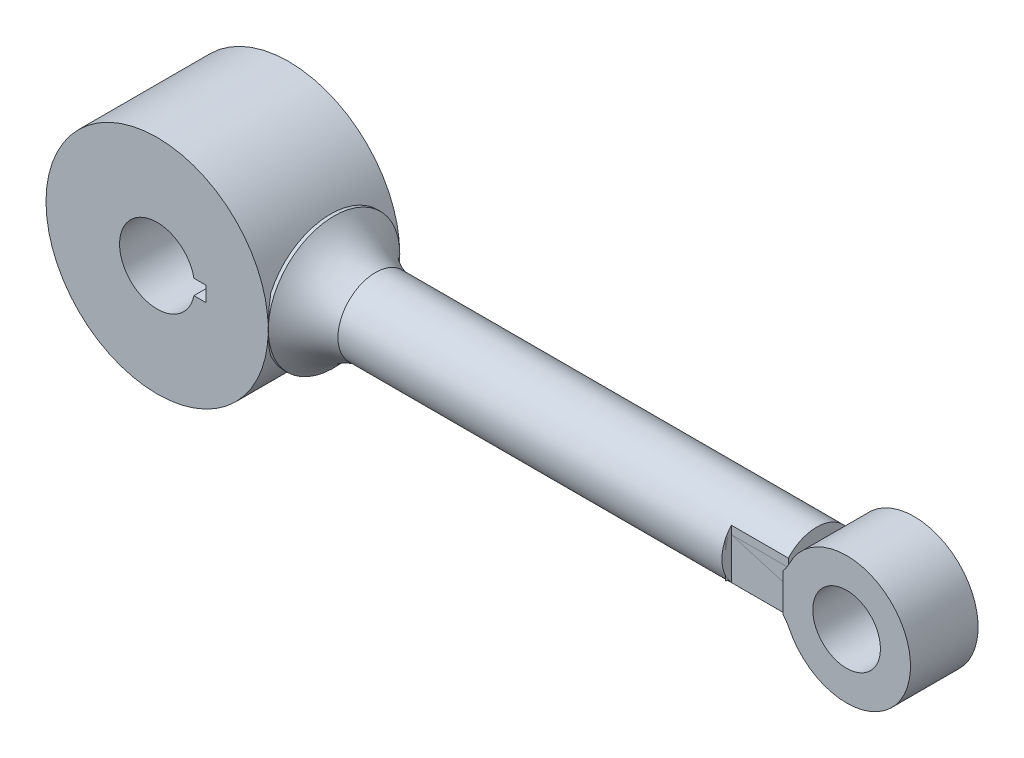
ISO-10303-21;
HEADER;
FILE_DESCRIPTION(('STEP AP214'),'2;1');
FILE_NAME('part.step','',(''),(''),'','','');
FILE_SCHEMA(('AUTOMOTIVE_DESIGN { 1 0 10303 214 1 1 1 1 }'));
ENDSEC;
DATA;
#1=APPLICATION_CONTEXT('core data for automotive mechanical design processes');
#2=APPLICATION_PROTOCOL_DEFINITION('international standard','automotive_design',2000,#1);
#3=PRODUCT_CONTEXT('',#1,'mechanical');
#4=PRODUCT('Part','Part','',(#3));
#5=PRODUCT_RELATED_PRODUCT_CATEGORY('part','',(#4));
#6=PRODUCT_DEFINITION_FORMATION('','',#4);
#7=PRODUCT_DEFINITION_CONTEXT('part definition',#1,'design');
#8=PRODUCT_DEFINITION('design','',#6,#7);
#9=PRODUCT_DEFINITION_SHAPE('','',#8);
#10=(LENGTH_UNIT() NAMED_UNIT(*) SI_UNIT(.MILLI.,.METRE.));
#11=(NAMED_UNIT(*) PLANE_ANGLE_UNIT() SI_UNIT($,.RADIAN.));
#12=(NAMED_UNIT(*) SI_UNIT($,.STERADIAN.) SOLID_ANGLE_UNIT());
#13=UNCERTAINTY_MEASURE_WITH_UNIT(LENGTH_MEASURE(1.E-05),#10,'distance_accuracy_value','');
#14=(GEOMETRIC_REPRESENTATION_CONTEXT(3) GLOBAL_UNCERTAINTY_ASSIGNED_CONTEXT((#13)) GLOBAL_UNIT_ASSIGNED_CONTEXT((#10,
#11,#12)) REPRESENTATION_CONTEXT('',''));
#15=CARTESIAN_POINT('',(0.,0.,0.));
#16=DIRECTION('',(0.,0.,1.));
#17=DIRECTION('',(1.,0.,0.));
#18=AXIS2_PLACEMENT_3D('',#15,#16,#17);
#19=CARTESIAN_POINT('',(0.,0.,9.));
#20=DIRECTION('',(0.,0.,1.));
#21=DIRECTION('',(1.,0.,0.));
#22=AXIS2_PLACEMENT_3D('',#19,#20,#21);
#23=PLANE('',#22);
#24=DIRECTION('',(0.,-1.,0.));
#25=VECTOR('',#24,1.);
#26=CARTESIAN_POINT('',(152.,0.,9.));
#27=LINE('',#26,#25);
#28=CARTESIAN_POINT('',(152.,4.44448924161109,9.));
#29=VERTEX_POINT('',#28);
#30=CARTESIAN_POINT('',(152.,-5.55551075838891,9.));
#31=VERTEX_POINT('',#30);
#32=EDGE_CURVE('E196',#29,#31,#27,.T.);
#33=ORIENTED_EDGE('',*,*,#32,.T.);
#34=CARTESIAN_POINT('',(144.747213525935,-12.4400650912145,9.));
#35=DIRECTION('',(0.,0.,1.));
#36=DIRECTION('',(1.,0.,0.));
#37=AXIS2_PLACEMENT_3D('',#34,#35,#36);
#38=CIRCLE('',#37,10.);
#39=CARTESIAN_POINT('',(153.726364566168,-8.03837830127917,9.));
#40=VERTEX_POINT('',#39);
#41=EDGE_CURVE('E203',#31,#40,#38,.F.);
#42=ORIENTED_EDGE('',*,*,#41,.T.);
#43=CARTESIAN_POINT('',(168.990921334563,-0.555510758389091,9.));
#44=DIRECTION('',(0.,0.,1.));
#45=DIRECTION('',(1.,0.,0.));
#46=AXIS2_PLACEMENT_3D('',#43,#44,#45);
#47=CIRCLE('',#46,17.);
#48=CARTESIAN_POINT('',(153.726364566168,6.92735678450099,9.));
#49=VERTEX_POINT('',#48);
#50=EDGE_CURVE('E210',#40,#49,#47,.T.);
#51=ORIENTED_EDGE('',*,*,#50,.T.);
#52=CARTESIAN_POINT('',(144.747213525935,11.3290435744363,9.));
#53=DIRECTION('',(0.,0.,1.));
#54=DIRECTION('',(1.,0.,0.));
#55=AXIS2_PLACEMENT_3D('',#52,#53,#54);
#56=CIRCLE('',#55,10.);
#57=EDGE_CURVE('E209',#29,#49,#56,.T.);
#58=ORIENTED_EDGE('',*,*,#57,.F.);
#59=EDGE_LOOP('',(#33,#42,#51,#58));
#60=FACE_BOUND('',#59,.T.);
#61=CARTESIAN_POINT('',(168.990921334563,-0.555510758389091,9.));
#62=DIRECTION('',(0.,0.,1.));
#63=DIRECTION('',(1.,0.,0.));
#64=AXIS2_PLACEMENT_3D('',#61,#62,#63);
#65=CIRCLE('',#64,9.00000000000001);
#66=CARTESIAN_POINT('',(177.990921334563,-0.555510758389091,9.));
#67=VERTEX_POINT('',#66);
#68=EDGE_CURVE('E201',#67,#67,#65,.T.);
#69=ORIENTED_EDGE('',*,*,#68,.F.);
#70=EDGE_LOOP('',(#69));
#71=FACE_BOUND('',#70,.T.);
#72=ADVANCED_FACE('F55',(#60,#71),#23,.T.);
#73=CARTESIAN_POINT('',(0.,0.,-9.));
#74=DIRECTION('',(0.,0.,1.));
#75=DIRECTION('',(1.,0.,0.));
#76=AXIS2_PLACEMENT_3D('',#73,#74,#75);
#77=PLANE('',#76);
#78=CARTESIAN_POINT('',(168.990921334563,-0.555510758389091,-9.));
#79=DIRECTION('',(0.,0.,1.));
#80=DIRECTION('',(1.,0.,0.));
#81=AXIS2_PLACEMENT_3D('',#78,#79,#80);
#82=CIRCLE('',#81,9.00000000000001);
#83=CARTESIAN_POINT('',(177.990921334563,-0.555510758389091,-9.));
#84=VERTEX_POINT('',#83);
#85=EDGE_CURVE('E221',#84,#84,#82,.T.);
#86=ORIENTED_EDGE('',*,*,#85,.T.);
#87=EDGE_LOOP('',(#86));
#88=FACE_BOUND('',#87,.T.);
#89=CARTESIAN_POINT('',(144.747213525935,-12.4400650912145,-9.));
#90=DIRECTION('',(0.,0.,1.));
#91=DIRECTION('',(1.,0.,0.));
#92=AXIS2_PLACEMENT_3D('',#89,#90,#91);
#93=CIRCLE('',#92,10.);
#94=CARTESIAN_POINT('',(152.,-5.55551075838891,-9.));
#95=VERTEX_POINT('',#94);
#96=CARTESIAN_POINT('',(153.726364566168,-8.03837830127917,-9.));
#97=VERTEX_POINT('',#96);
#98=EDGE_CURVE('E223',#95,#97,#93,.F.);
#99=ORIENTED_EDGE('',*,*,#98,.F.);
#100=DIRECTION('',(0.,-1.,0.));
#101=VECTOR('',#100,1.);
#102=CARTESIAN_POINT('',(152.,0.,-9.));
#103=LINE('',#102,#101);
#104=CARTESIAN_POINT('',(152.,4.4444892416109,-9.));
#105=VERTEX_POINT('',#104);
#106=EDGE_CURVE('E199',#105,#95,#103,.T.);
#107=ORIENTED_EDGE('',*,*,#106,.F.);
#108=CARTESIAN_POINT('',(144.747213525935,11.3290435744363,-9.));
#109=DIRECTION('',(0.,0.,1.));
#110=DIRECTION('',(1.,0.,0.));
#111=AXIS2_PLACEMENT_3D('',#108,#109,#110);
#112=CIRCLE('',#111,10.);
#113=CARTESIAN_POINT('',(153.726364566168,6.92735678450099,-9.));
#114=VERTEX_POINT('',#113);
#115=EDGE_CURVE('E229',#105,#114,#112,.T.);
#116=ORIENTED_EDGE('',*,*,#115,.T.);
#117=CARTESIAN_POINT('',(168.990921334563,-0.555510758389091,-9.));
#118=DIRECTION('',(0.,0.,1.));
#119=DIRECTION('',(1.,0.,0.));
#120=AXIS2_PLACEMENT_3D('',#117,#118,#119);
#121=CIRCLE('',#120,17.);
#122=EDGE_CURVE('E227',#97,#114,#121,.T.);
#123=ORIENTED_EDGE('',*,*,#122,.F.);
#124=EDGE_LOOP('',(#99,#107,#116,#123));
#125=FACE_BOUND('',#124,.T.);
#126=ADVANCED_FACE('F296',(#88,#125),#77,.F.);
#127=CARTESIAN_POINT('',(144.747213525935,-12.4400650912145,9.));
#128=DIRECTION('',(0.,0.,-1.));
#129=DIRECTION('',(-1.,0.,0.));
#130=AXIS2_PLACEMENT_3D('',#127,#128,#129);
#131=CYLINDRICAL_SURFACE('',#130,10.);
#132=ORIENTED_EDGE('',*,*,#98,.T.);
#133=DIRECTION('',(0.,0.,-1.));
#134=VECTOR('',#133,1.);
#135=CARTESIAN_POINT('',(153.726364566168,-8.03837830127917,9.));
#136=LINE('',#135,#134);
#137=EDGE_CURVE('E254',#40,#97,#136,.T.);
#138=ORIENTED_EDGE('',*,*,#137,.F.);
#139=ORIENTED_EDGE('',*,*,#41,.F.);
#140=DIRECTION('',(0.,0.,-1.));
#141=VECTOR('',#140,1.);
#142=CARTESIAN_POINT('',(152.,-5.55551075838909,9.));
#143=LINE('',#142,#141);
#144=CARTESIAN_POINT('',(152.,-5.55551075838891,7.50568973264478));
#145=VERTEX_POINT('',#144);
#146=EDGE_CURVE('E237',#31,#145,#143,.T.);
#147=ORIENTED_EDGE('',*,*,#146,.T.);
#148=CARTESIAN_POINT('',(152.,-5.55551075838891,-7.44583228498236));
#149=VERTEX_POINT('',#148);
#150=EDGE_CURVE('E243',#145,#149,#143,.T.);
#151=ORIENTED_EDGE('',*,*,#150,.T.);
#152=DIRECTION('',(0.,0.,1.));
#153=VECTOR('',#152,1.);
#154=CARTESIAN_POINT('',(152.,-5.55551075838909,9.));
#155=LINE('',#154,#153);
#156=EDGE_CURVE('E176',#95,#149,#155,.T.);
#157=ORIENTED_EDGE('',*,*,#156,.F.);
#158=EDGE_LOOP('',(#132,#138,#139,#147,#151,#157));
#159=FACE_BOUND('',#158,.T.);
#160=ADVANCED_FACE('F301',(#159),#131,.F.);
#161=CARTESIAN_POINT('',(168.990921334563,-0.555510758389091,9.));
#162=DIRECTION('',(0.,0.,-1.));
#163=DIRECTION('',(-1.,0.,0.));
#164=AXIS2_PLACEMENT_3D('',#161,#162,#163);
#165=CYLINDRICAL_SURFACE('',#164,17.);
#166=ORIENTED_EDGE('',*,*,#122,.T.);
#167=DIRECTION('',(0.,0.,-1.));
#168=VECTOR('',#167,1.);
#169=CARTESIAN_POINT('',(153.726364566168,6.92735678450099,9.));
#170=LINE('',#169,#168);
#171=EDGE_CURVE('E252',#49,#114,#170,.T.);
#172=ORIENTED_EDGE('',*,*,#171,.F.);
#173=ORIENTED_EDGE('',*,*,#50,.F.);
#174=ORIENTED_EDGE('',*,*,#137,.T.);
#175=EDGE_LOOP('',(#166,#172,#173,#174));
#176=FACE_BOUND('',#175,.T.);
#177=ADVANCED_FACE('F320',(#176),#165,.T.);
#178=CARTESIAN_POINT('',(144.747213525935,11.3290435744363,9.));
#179=DIRECTION('',(0.,0.,-1.));
#180=DIRECTION('',(-1.,0.,0.));
#181=AXIS2_PLACEMENT_3D('',#178,#179,#180);
#182=CYLINDRICAL_SURFACE('',#181,10.);
#183=ORIENTED_EDGE('',*,*,#115,.F.);
#184=DIRECTION('',(0.,0.,1.));
#185=VECTOR('',#184,1.);
#186=CARTESIAN_POINT('',(152.,4.44448924161091,9.));
#187=LINE('',#186,#185);
#188=CARTESIAN_POINT('',(152.,4.44448924161109,-7.44583228498236));
#189=VERTEX_POINT('',#188);
#190=EDGE_CURVE('E182',#105,#189,#187,.T.);
#191=ORIENTED_EDGE('',*,*,#190,.T.);
#192=DIRECTION('',(0.,0.,-1.));
#193=VECTOR('',#192,1.);
#194=CARTESIAN_POINT('',(152.,4.44448924161109,9.));
#195=LINE('',#194,#193);
#196=CARTESIAN_POINT('',(152.,4.44448924161109,7.50568973264478));
#197=VERTEX_POINT('',#196);
#198=EDGE_CURVE('E247',#197,#189,#195,.T.);
#199=ORIENTED_EDGE('',*,*,#198,.F.);
#200=EDGE_CURVE('E248',#29,#197,#195,.T.);
#201=ORIENTED_EDGE('',*,*,#200,.F.);
#202=ORIENTED_EDGE('',*,*,#57,.T.);
#203=ORIENTED_EDGE('',*,*,#171,.T.);
#204=EDGE_LOOP('',(#183,#191,#199,#201,#202,#203));
#205=FACE_BOUND('',#204,.T.);
#206=ADVANCED_FACE('F291',(#205),#182,.F.);
#207=CARTESIAN_POINT('',(1.07845184439105E-13,4.4444892416146,9.));
#208=DIRECTION('',(0.,-1.,0.));
#209=DIRECTION('',(1.,0.,0.));
#210=AXIS2_PLACEMENT_3D('',#207,#208,#209);
#211=PLANE('',#210);
#212=DIRECTION('',(-1.,0.,0.));
#213=VECTOR('',#212,1.);
#214=CARTESIAN_POINT('',(1.07845184439105E-13,4.4444892416146,9.));
#215=LINE('',#214,#213);
#216=CARTESIAN_POINT('',(136.808358121643,4.44448924161128,9.));
#217=VERTEX_POINT('',#216);
#218=CARTESIAN_POINT('',(136.80816300163,4.44448924161128,9.));
#219=VERTEX_POINT('',#218);
#220=EDGE_CURVE('E215',#217,#219,#215,.T.);
#221=ORIENTED_EDGE('',*,*,#220,.F.);
#222=DIRECTION('',(0.,0.,-1.));
#223=VECTOR('',#222,1.);
#224=CARTESIAN_POINT('',(136.808358121643,4.44448924161128,9.));
#225=LINE('',#224,#223);
#226=CARTESIAN_POINT('',(136.808358121643,4.44448924161109,7.50568973264478));
#227=VERTEX_POINT('',#226);
#228=EDGE_CURVE('E70',#217,#227,#225,.T.);
#229=ORIENTED_EDGE('',*,*,#228,.T.);
#230=DIRECTION('',(1.,0.,0.));
#231=VECTOR('',#230,1.);
#232=CARTESIAN_POINT('',(1.07845184439105E-13,4.4444892416146,7.50568973264478));
#233=LINE('',#232,#231);
#234=EDGE_CURVE('E194',#227,#197,#233,.T.);
#235=ORIENTED_EDGE('',*,*,#234,.T.);
#236=ORIENTED_EDGE('',*,*,#198,.T.);
#237=DIRECTION('',(-1.,0.,0.));
#238=VECTOR('',#237,1.);
#239=CARTESIAN_POINT('',(1.07845184439105E-13,4.4444892416146,-7.44583228498236));
#240=LINE('',#239,#238);
#241=CARTESIAN_POINT('',(136.808358121643,4.44448924161128,-7.44583228498236));
#242=VERTEX_POINT('',#241);
#243=EDGE_CURVE('E191',#189,#242,#240,.T.);
#244=ORIENTED_EDGE('',*,*,#243,.T.);
#245=DIRECTION('',(0.,0.,-1.));
#246=VECTOR('',#245,1.);
#247=CARTESIAN_POINT('',(136.808358121643,4.44448924161128,9.));
#248=LINE('',#247,#246);
#249=CARTESIAN_POINT('',(136.808358121643,4.44448924161118,-9.));
#250=VERTEX_POINT('',#249);
#251=EDGE_CURVE('E168',#242,#250,#248,.T.);
#252=ORIENTED_EDGE('',*,*,#251,.T.);
#253=DIRECTION('',(-1.,0.,0.));
#254=VECTOR('',#253,1.);
#255=CARTESIAN_POINT('',(1.07845184439105E-13,4.4444892416146,-9.));
#256=LINE('',#255,#254);
#257=CARTESIAN_POINT('',(136.80816300163,4.44448924161128,-9.));
#258=VERTEX_POINT('',#257);
#259=EDGE_CURVE('E231',#250,#258,#256,.T.);
#260=ORIENTED_EDGE('',*,*,#259,.T.);
#261=DIRECTION('',(0.,0.,-1.));
#262=VECTOR('',#261,1.);
#263=CARTESIAN_POINT('',(136.80816300163,4.44448924161128,9.));
#264=LINE('',#263,#262);
#265=EDGE_CURVE('E244',#219,#258,#264,.T.);
#266=ORIENTED_EDGE('',*,*,#265,.F.);
#267=EDGE_LOOP('',(#221,#229,#235,#236,#244,#252,#260,#266));
#268=FACE_BOUND('',#267,.T.);
#269=ADVANCED_FACE('F279',(#268),#211,.F.);
#270=CARTESIAN_POINT('',(136.80816300163,0.,9.));
#271=DIRECTION('',(-1.,0.,0.));
#272=DIRECTION('',(0.,0.,1.));
#273=AXIS2_PLACEMENT_3D('',#270,#271,#272);
#274=PLANE('',#273);
#275=DIRECTION('',(0.,1.,0.));
#276=VECTOR('',#275,1.);
#277=CARTESIAN_POINT('',(136.80816300163,0.,-9.));
#278=LINE('',#277,#276);
#279=CARTESIAN_POINT('',(136.80816300163,-5.55551075838872,-9.));
#280=VERTEX_POINT('',#279);
#281=EDGE_CURVE('E232',#280,#258,#278,.T.);
#282=ORIENTED_EDGE('',*,*,#281,.F.);
#283=DIRECTION('',(0.,0.,-1.));
#284=VECTOR('',#283,1.);
#285=CARTESIAN_POINT('',(136.80816300163,-5.55551075838872,9.));
#286=LINE('',#285,#284);
#287=CARTESIAN_POINT('',(136.80816300163,-5.55551075838872,9.));
#288=VERTEX_POINT('',#287);
#289=EDGE_CURVE('E245',#288,#280,#286,.T.);
#290=ORIENTED_EDGE('',*,*,#289,.F.);
#291=DIRECTION('',(0.,1.,0.));
#292=VECTOR('',#291,1.);
#293=CARTESIAN_POINT('',(136.80816300163,0.,9.));
#294=LINE('',#293,#292);
#295=EDGE_CURVE('E213',#288,#219,#294,.T.);
#296=ORIENTED_EDGE('',*,*,#295,.T.);
#297=ORIENTED_EDGE('',*,*,#265,.T.);
#298=EDGE_LOOP('',(#282,#290,#296,#297));
#299=FACE_BOUND('',#298,.T.);
#300=ADVANCED_FACE('F273',(#299),#274,.T.);
#301=CARTESIAN_POINT('',(168.990921334563,-0.555510758389091,9.));
#302=DIRECTION('',(0.,0.,-1.));
#303=DIRECTION('',(-1.,0.,0.));
#304=AXIS2_PLACEMENT_3D('',#301,#302,#303);
#305=CYLINDRICAL_SURFACE('',#304,17.);
#306=CARTESIAN_POINT('',(168.990921334563,-0.555510758389091,7.50568973264478));
#307=DIRECTION('',(0.,0.,-1.));
#308=DIRECTION('',(-1.,0.,0.));
#309=AXIS2_PLACEMENT_3D('',#306,#307,#308);
#310=CIRCLE('',#309,17.);
#311=CARTESIAN_POINT('',(152.,-1.11102151677812,7.50568973264478));
#312=VERTEX_POINT('',#311);
#313=CARTESIAN_POINT('',(152.,0.,7.50568973264478));
#314=VERTEX_POINT('',#313);
#315=EDGE_CURVE('E192',#312,#314,#310,.T.);
#316=ORIENTED_EDGE('',*,*,#315,.F.);
#317=DIRECTION('',(0.,0.,-1.));
#318=VECTOR('',#317,1.);
#319=CARTESIAN_POINT('',(152.,-1.11102151677812,9.));
#320=LINE('',#319,#318);
#321=CARTESIAN_POINT('',(152.,-1.11102151677812,-7.44583228498236));
#322=VERTEX_POINT('',#321);
#323=EDGE_CURVE('E216',#312,#322,#320,.T.);
#324=ORIENTED_EDGE('',*,*,#323,.T.);
#325=CARTESIAN_POINT('',(168.990921334563,-0.555510758389091,-7.44583228498236));
#326=DIRECTION('',(0.,0.,1.));
#327=DIRECTION('',(1.,0.,0.));
#328=AXIS2_PLACEMENT_3D('',#325,#326,#327);
#329=CIRCLE('',#328,17.);
#330=CARTESIAN_POINT('',(152.,0.,-7.44583228498236));
#331=VERTEX_POINT('',#330);
#332=EDGE_CURVE('E186',#331,#322,#329,.T.);
#333=ORIENTED_EDGE('',*,*,#332,.F.);
#334=DIRECTION('',(0.,0.,-1.));
#335=VECTOR('',#334,1.);
#336=CARTESIAN_POINT('',(152.,0.,9.));
#337=LINE('',#336,#335);
#338=EDGE_CURVE('E258',#314,#331,#337,.T.);
#339=ORIENTED_EDGE('',*,*,#338,.F.);
#340=EDGE_LOOP('',(#316,#324,#333,#339));
#341=FACE_BOUND('',#340,.T.);
#342=ADVANCED_FACE('F53',(#341),#305,.F.);
#343=CARTESIAN_POINT('',(168.990921334563,-0.555510758389091,9.));
#344=DIRECTION('',(0.,0.,-1.));
#345=DIRECTION('',(-1.,0.,0.));
#346=AXIS2_PLACEMENT_3D('',#343,#344,#345);
#347=CYLINDRICAL_SURFACE('',#346,9.00000000000001);
#348=ORIENTED_EDGE('',*,*,#68,.T.);
#349=EDGE_LOOP('',(#348));
#350=FACE_BOUND('',#349,.T.);
#351=ORIENTED_EDGE('',*,*,#85,.F.);
#352=EDGE_LOOP('',(#351));
#353=FACE_BOUND('',#352,.T.);
#354=ADVANCED_FACE('F344',(#350,#353),#347,.F.);
#355=CARTESIAN_POINT('',(152.,0.,9.));
#356=DIRECTION('',(1.,0.,0.));
#357=DIRECTION('',(0.,0.,-1.));
#358=AXIS2_PLACEMENT_3D('',#355,#356,#357);
#359=PLANE('',#358);
#360=ORIENTED_EDGE('',*,*,#323,.F.);
#361=DIRECTION('',(0.,1.,0.));
#362=VECTOR('',#361,1.);
#363=CARTESIAN_POINT('',(152.,-29.5745759677554,7.50568973264478));
#364=LINE('',#363,#362);
#365=EDGE_CURVE('E178',#145,#312,#364,.T.);
#366=ORIENTED_EDGE('',*,*,#365,.F.);
#367=ORIENTED_EDGE('',*,*,#146,.F.);
#368=ORIENTED_EDGE('',*,*,#32,.F.);
#369=ORIENTED_EDGE('',*,*,#200,.T.);
#370=EDGE_CURVE('E308',#314,#197,#364,.T.);
#371=ORIENTED_EDGE('',*,*,#370,.F.);
#372=ORIENTED_EDGE('',*,*,#338,.T.);
#373=DIRECTION('',(0.,1.,0.));
#374=VECTOR('',#373,1.);
#375=CARTESIAN_POINT('',(152.,-29.5745759677554,-7.44583228498236));
#376=LINE('',#375,#374);
#377=EDGE_CURVE('E170',#331,#189,#376,.T.);
#378=ORIENTED_EDGE('',*,*,#377,.T.);
#379=ORIENTED_EDGE('',*,*,#190,.F.);
#380=ORIENTED_EDGE('',*,*,#106,.T.);
#381=ORIENTED_EDGE('',*,*,#156,.T.);
#382=EDGE_CURVE('E158',#149,#322,#376,.T.);
#383=ORIENTED_EDGE('',*,*,#382,.T.);
#384=EDGE_LOOP('',(#360,#366,#367,#368,#369,#371,#372,#378,#379,#380,#381,#383));
#385=FACE_BOUND('',#384,.T.);
#386=ADVANCED_FACE('F287',(#385),#359,.F.);
#387=CARTESIAN_POINT('',(-1.35438406727716E-13,-5.55551075838539,9.));
#388=DIRECTION('',(0.,-1.,0.));
#389=DIRECTION('',(1.,0.,0.));
#390=AXIS2_PLACEMENT_3D('',#387,#388,#389);
#391=PLANE('',#390);
#392=DIRECTION('',(0.,0.,-1.));
#393=VECTOR('',#392,1.);
#394=CARTESIAN_POINT('',(136.808358121643,-5.55551075838872,9.));
#395=LINE('',#394,#393);
#396=CARTESIAN_POINT('',(136.808358121643,-5.55551075838891,9.));
#397=VERTEX_POINT('',#396);
#398=CARTESIAN_POINT('',(136.808358121643,-5.55551075838891,7.50568973264478));
#399=VERTEX_POINT('',#398);
#400=EDGE_CURVE('E187',#397,#399,#395,.T.);
#401=ORIENTED_EDGE('',*,*,#400,.F.);
#402=DIRECTION('',(-1.,0.,0.));
#403=VECTOR('',#402,1.);
#404=CARTESIAN_POINT('',(-1.35438406727716E-13,-5.55551075838539,9.));
#405=LINE('',#404,#403);
#406=EDGE_CURVE('E220',#397,#288,#405,.T.);
#407=ORIENTED_EDGE('',*,*,#406,.T.);
#408=ORIENTED_EDGE('',*,*,#289,.T.);
#409=DIRECTION('',(-1.,0.,0.));
#410=VECTOR('',#409,1.);
#411=CARTESIAN_POINT('',(-1.35438406727716E-13,-5.55551075838539,-9.));
#412=LINE('',#411,#410);
#413=CARTESIAN_POINT('',(136.808358121643,-5.55551075838872,-9.));
#414=VERTEX_POINT('',#413);
#415=EDGE_CURVE('E173',#414,#280,#412,.T.);
#416=ORIENTED_EDGE('',*,*,#415,.F.);
#417=DIRECTION('',(0.,0.,-1.));
#418=VECTOR('',#417,1.);
#419=CARTESIAN_POINT('',(136.808358121643,-5.55551075838872,9.));
#420=LINE('',#419,#418);
#421=CARTESIAN_POINT('',(136.808358121643,-5.55551075838872,-7.44583228498236));
#422=VERTEX_POINT('',#421);
#423=EDGE_CURVE('E74',#422,#414,#420,.T.);
#424=ORIENTED_EDGE('',*,*,#423,.F.);
#425=DIRECTION('',(-1.,0.,0.));
#426=VECTOR('',#425,1.);
#427=CARTESIAN_POINT('',(-1.35438406727716E-13,-5.55551075838539,-7.44583228498236));
#428=LINE('',#427,#426);
#429=EDGE_CURVE('E58',#149,#422,#428,.T.);
#430=ORIENTED_EDGE('',*,*,#429,.F.);
#431=ORIENTED_EDGE('',*,*,#150,.F.);
#432=DIRECTION('',(1.,0.,0.));
#433=VECTOR('',#432,1.);
#434=CARTESIAN_POINT('',(-1.35438406727716E-13,-5.55551075838539,7.50568973264478));
#435=LINE('',#434,#433);
#436=EDGE_CURVE('E12',#399,#145,#435,.T.);
#437=ORIENTED_EDGE('',*,*,#436,.F.);
#438=EDGE_LOOP('',(#401,#407,#408,#416,#424,#430,#431,#437));
#439=FACE_BOUND('',#438,.T.);
#440=ADVANCED_FACE('F171',(#439),#391,.T.);
#441=DIRECTION('',(0.,-1.,0.));
#442=VECTOR('',#441,1.);
#443=CARTESIAN_POINT('',(136.808358121643,0.,9.));
#444=LINE('',#443,#442);
#445=EDGE_CURVE('E161',#217,#397,#444,.T.);
#446=ORIENTED_EDGE('',*,*,#445,.F.);
#447=ORIENTED_EDGE('',*,*,#220,.T.);
#448=ORIENTED_EDGE('',*,*,#295,.F.);
#449=ORIENTED_EDGE('',*,*,#406,.F.);
#450=EDGE_LOOP('',(#446,#447,#448,#449));
#451=FACE_BOUND('',#450,.T.);
#452=ADVANCED_FACE('F272',(#451),#23,.T.);
#453=ORIENTED_EDGE('',*,*,#259,.F.);
#454=DIRECTION('',(0.,-1.,0.));
#455=VECTOR('',#454,1.);
#456=CARTESIAN_POINT('',(136.808358121643,0.,-9.));
#457=LINE('',#456,#455);
#458=EDGE_CURVE('E256',#250,#414,#457,.T.);
#459=ORIENTED_EDGE('',*,*,#458,.T.);
#460=ORIENTED_EDGE('',*,*,#415,.T.);
#461=ORIENTED_EDGE('',*,*,#281,.T.);
#462=EDGE_LOOP('',(#453,#459,#460,#461));
#463=FACE_BOUND('',#462,.T.);
#464=ADVANCED_FACE('F277',(#463),#77,.F.);
#465=CARTESIAN_POINT('',(152.,-29.5745759677554,-7.44583228498236));
#466=DIRECTION('',(0.,0.,1.));
#467=DIRECTION('',(1.,0.,0.));
#468=AXIS2_PLACEMENT_3D('',#465,#466,#467);
#469=PLANE('',#468);
#470=ORIENTED_EDGE('',*,*,#377,.F.);
#471=ORIENTED_EDGE('',*,*,#332,.T.);
#472=ORIENTED_EDGE('',*,*,#382,.F.);
#473=ORIENTED_EDGE('',*,*,#429,.T.);
#474=DIRECTION('',(0.,1.,0.));
#475=VECTOR('',#474,1.);
#476=CARTESIAN_POINT('',(136.808358121643,-29.5745759677554,-7.44583228498236));
#477=LINE('',#476,#475);
#478=EDGE_CURVE('E156',#422,#242,#477,.T.);
#479=ORIENTED_EDGE('',*,*,#478,.T.);
#480=ORIENTED_EDGE('',*,*,#243,.F.);
#481=EDGE_LOOP('',(#470,#471,#472,#473,#479,#480));
#482=FACE_BOUND('',#481,.T.);
#483=ADVANCED_FACE('F153',(#482),#469,.F.);
#484=CARTESIAN_POINT('',(136.808358121643,-29.5745759677554,-7.44583228498236));
#485=DIRECTION('',(-1.,0.,0.));
#486=DIRECTION('',(0.,0.,1.));
#487=AXIS2_PLACEMENT_3D('',#484,#485,#486);
#488=PLANE('',#487);
#489=ORIENTED_EDGE('',*,*,#478,.F.);
#490=ORIENTED_EDGE('',*,*,#423,.T.);
#491=ORIENTED_EDGE('',*,*,#458,.F.);
#492=ORIENTED_EDGE('',*,*,#251,.F.);
#493=EDGE_LOOP('',(#489,#490,#491,#492));
#494=FACE_BOUND('',#493,.T.);
#495=ADVANCED_FACE('F165',(#494),#488,.F.);
#496=CARTESIAN_POINT('',(152.,-29.5745759677554,7.50568973264478));
#497=DIRECTION('',(0.,0.,-1.));
#498=DIRECTION('',(-1.,0.,0.));
#499=AXIS2_PLACEMENT_3D('',#496,#497,#498);
#500=PLANE('',#499);
#501=DIRECTION('',(0.,1.,0.));
#502=VECTOR('',#501,1.);
#503=CARTESIAN_POINT('',(136.808358121643,-29.5745759677554,7.50568973264478));
#504=LINE('',#503,#502);
#505=EDGE_CURVE('E172',#399,#227,#504,.T.);
#506=ORIENTED_EDGE('',*,*,#505,.F.);
#507=ORIENTED_EDGE('',*,*,#436,.T.);
#508=ORIENTED_EDGE('',*,*,#365,.T.);
#509=ORIENTED_EDGE('',*,*,#315,.T.);
#510=ORIENTED_EDGE('',*,*,#370,.T.);
#511=ORIENTED_EDGE('',*,*,#234,.F.);
#512=EDGE_LOOP('',(#506,#507,#508,#509,#510,#511));
#513=FACE_BOUND('',#512,.T.);
#514=ADVANCED_FACE('F315',(#513),#500,.F.);
#515=CARTESIAN_POINT('',(136.808358121643,-29.5745759677554,7.50568973264478));
#516=DIRECTION('',(-1.,0.,0.));
#517=DIRECTION('',(0.,0.,1.));
#518=AXIS2_PLACEMENT_3D('',#515,#516,#517);
#519=PLANE('',#518);
#520=ORIENTED_EDGE('',*,*,#445,.T.);
#521=ORIENTED_EDGE('',*,*,#400,.T.);
#522=ORIENTED_EDGE('',*,*,#505,.T.);
#523=ORIENTED_EDGE('',*,*,#228,.F.);
#524=EDGE_LOOP('',(#520,#521,#522,#523));
#525=FACE_BOUND('',#524,.T.);
#526=ADVANCED_FACE('F264',(#525),#519,.F.);
#527=CLOSED_SHELL('',(#72,#126,#160,#177,#206,#269,#300,#342,#354,#386,#440,#452,#464,#483,#495,
#514,#526));
#528=MANIFOLD_SOLID_BREP('B2',#527);
#529=CARTESIAN_POINT('',(-6.,0.,17.5));
#530=DIRECTION('',(0.,0.,-1.));
#531=DIRECTION('',(-1.,0.,0.));
#532=AXIS2_PLACEMENT_3D('',#529,#530,#531);
#533=CYLINDRICAL_SURFACE('',#532,29.5745759677554);
#534=CARTESIAN_POINT('',(-6.,0.,-17.5));
#535=DIRECTION('',(0.,0.,1.));
#536=DIRECTION('',(1.,0.,0.));
#537=AXIS2_PLACEMENT_3D('',#534,#535,#536);
#538=CIRCLE('',#537,29.5745759677554);
#539=CARTESIAN_POINT('',(23.5745759677554,0.,-17.5));
#540=VERTEX_POINT('',#539);
#541=EDGE_CURVE('E571',#540,#540,#538,.T.);
#542=ORIENTED_EDGE('',*,*,#541,.T.);
#543=EDGE_LOOP('',(#542));
#544=FACE_BOUND('',#543,.T.);
#545=CARTESIAN_POINT('',(-6.,0.,17.5));
#546=DIRECTION('',(0.,0.,1.));
#547=DIRECTION('',(1.,0.,0.));
#548=AXIS2_PLACEMENT_3D('',#545,#546,#547);
#549=CIRCLE('',#548,29.5745759677554);
#550=CARTESIAN_POINT('',(23.5745759677554,0.,17.5));
#551=VERTEX_POINT('',#550);
#552=EDGE_CURVE('E558',#551,#551,#549,.T.);
#553=ORIENTED_EDGE('',*,*,#552,.F.);
#554=EDGE_LOOP('',(#553));
#555=FACE_BOUND('',#554,.T.);
#556=CARTESIAN_POINT('',(-35.5745759677554,0.,4.));
#557=CARTESIAN_POINT('',(-35.5745726464188,0.223587053881961,3.99999060204183));
#558=CARTESIAN_POINT('',(-35.5720137550307,0.44730995803308,3.98119006957602));
#559=CARTESIAN_POINT('',(-35.5620520169089,0.888519462414035,3.9064939956445));
#560=CARTESIAN_POINT('',(-35.5546442448937,1.10599948668054,3.85056073554996));
#561=CARTESIAN_POINT('',(-35.5358184726075,1.52827280908149,3.70328659676054));
#562=CARTESIAN_POINT('',(-35.5244033017846,1.73307493881647,3.61197069548615));
#563=CARTESIAN_POINT('',(-35.4988291253498,2.12441239444769,3.39658061497538));
#564=CARTESIAN_POINT('',(-35.4846705554836,2.31095061420448,3.27251163691602));
#565=CARTESIAN_POINT('',(-35.4550865344889,2.66169560859799,2.99428907298905));
#566=CARTESIAN_POINT('',(-35.4396542987345,2.8257685151112,2.83996742849576));
#567=CARTESIAN_POINT('',(-35.4093163284954,3.12577169368954,2.50598142492202));
#568=CARTESIAN_POINT('',(-35.3944106221673,3.26170046259973,2.32631571309721));
#569=CARTESIAN_POINT('',(-35.3667470993739,3.50206465610198,1.94585963171566));
#570=CARTESIAN_POINT('',(-35.3539980388187,3.60637299800852,1.74498828233236));
#571=CARTESIAN_POINT('',(-35.3321822025942,3.77972363187251,1.32837739304229));
#572=CARTESIAN_POINT('',(-35.3231152638038,3.84876748611083,1.11263851227481));
#573=CARTESIAN_POINT('',(-35.3097559315649,3.94921878261714,0.673813854518597));
#574=CARTESIAN_POINT('',(-35.3054347054198,3.98085359565231,0.450781018295045));
#575=CARTESIAN_POINT('',(-35.3019681454803,4.00629269562973,0.00253357674892736));
#576=CARTESIAN_POINT('',(-35.3028225691156,4.0000987555155,-0.222680925830203));
#577=CARTESIAN_POINT('',(-35.3095843862257,3.95024248783192,-0.667305769239957));
#578=CARTESIAN_POINT('',(-35.3154578578205,3.90683168876754,-0.88674490381784));
#579=CARTESIAN_POINT('',(-35.3315430465176,3.78416692614975,-1.31519521923504));
#580=CARTESIAN_POINT('',(-35.3417548651545,3.70491212370074,-1.52420615588495));
#581=CARTESIAN_POINT('',(-35.3654042215841,3.5125421674881,-1.92664215762881));
#582=CARTESIAN_POINT('',(-35.3788520420162,3.39931878715602,-2.12001485997739));
#583=CARTESIAN_POINT('',(-35.4074504417505,3.14230295438681,-2.48511108739648));
#584=CARTESIAN_POINT('',(-35.4226011121156,2.99850886676074,-2.65683345363454));
#585=CARTESIAN_POINT('',(-35.4530485718421,2.68304458810284,-2.97521355981328));
#586=CARTESIAN_POINT('',(-35.4683455498241,2.51115780181857,-3.12165675541483));
#587=CARTESIAN_POINT('',(-35.4972474428745,2.14513017569803,-3.38364740891453));
#588=CARTESIAN_POINT('',(-35.5108523528188,1.95098926847395,-3.49919477325335));
#589=CARTESIAN_POINT('',(-35.5348477690872,1.5457909318595,-3.6961181620276));
#590=CARTESIAN_POINT('',(-35.5452368973709,1.33472629888535,-3.7774795422632));
#591=CARTESIAN_POINT('',(-35.5616181199173,0.901758591950915,-3.90354482521341));
#592=CARTESIAN_POINT('',(-35.5676104554325,0.679856113377063,-3.94825073923313));
#593=CARTESIAN_POINT('',(-35.57449133558,0.233365437919482,-3.99945518543063));
#594=CARTESIAN_POINT('',(-35.5754193272464,0.0088116926870187,-4.00624903054324));
#595=CARTESIAN_POINT('',(-35.5721738057196,-0.438231379464094,-3.98221757655431));
#596=CARTESIAN_POINT('',(-35.568000420201,-0.660720757908248,-3.95139321894208));
#597=CARTESIAN_POINT('',(-35.5550455474641,-1.09643907053862,-3.85324578969901));
#598=CARTESIAN_POINT('',(-35.5462819928699,-1.30970057015563,-3.78606472081673));
#599=CARTESIAN_POINT('',(-35.5251271824928,-1.72193145569186,-3.61725934748225));
#600=CARTESIAN_POINT('',(-35.5127357847131,-1.9209002818041,-3.51563369481546));
#601=CARTESIAN_POINT('',(-35.4856066857169,-2.30020885130901,-3.28011788007848));
#602=CARTESIAN_POINT('',(-35.4708553764499,-2.48042988375082,-3.14603812398417));
#603=CARTESIAN_POINT('',(-35.4406960437679,-2.81591640231137,-2.84968668779032));
#604=CARTESIAN_POINT('',(-35.4252879896625,-2.97118072055117,-2.68741368909369));
#605=CARTESIAN_POINT('',(-35.3954287118421,-3.25340465280172,-2.33797576081166));
#606=CARTESIAN_POINT('',(-35.3809845913501,-3.38016763479915,-2.15065132426318));
#607=CARTESIAN_POINT('',(-35.3548089806899,-3.6004289160371,-1.75719613880699));
#608=CARTESIAN_POINT('',(-35.343077428503,-3.69392797583142,-1.55106582001661));
#609=CARTESIAN_POINT('',(-35.3237049096792,-3.84469421808821,-1.12646585877276));
#610=CARTESIAN_POINT('',(-35.3160517623382,-3.90206938362638,-0.908035138538229));
#611=CARTESIAN_POINT('',(-35.3056686638407,-3.97930543762524,-0.464528494820006));
#612=CARTESIAN_POINT('',(-35.3029384410805,-3.99916839568389,-0.239452938636573));
#613=CARTESIAN_POINT('',(-35.3027191275013,-4.00077383676595,0.208996791782667));
#614=CARTESIAN_POINT('',(-35.3051875535789,-3.98282531302117,0.432369901400604));
#615=CARTESIAN_POINT('',(-35.3149956896481,-3.90997465333573,0.872892022922595));
#616=CARTESIAN_POINT('',(-35.3223353972166,-3.85507253577715,1.09004103792269));
#617=CARTESIAN_POINT('',(-35.3410452895633,-3.70997479582011,1.5118926428178));
#618=CARTESIAN_POINT('',(-35.3524134731271,-3.61979669506243,1.71660135360182));
#619=CARTESIAN_POINT('',(-35.3779023464429,-3.40673719392825,2.10803215917576));
#620=CARTESIAN_POINT('',(-35.3920230937685,-3.28385510948431,2.29475387762147));
#621=CARTESIAN_POINT('',(-35.4215640090331,-3.00773825938129,2.64648644491595));
#622=CARTESIAN_POINT('',(-35.4369934744078,-2.85427366388889,2.81131610806511));
#623=CARTESIAN_POINT('',(-35.4673329258534,-2.52183143130662,3.11299769232201));
#624=CARTESIAN_POINT('',(-35.4822427893506,-2.34284782432708,3.249843048525));
#625=CARTESIAN_POINT('',(-35.5099374823227,-1.96352442358531,3.49220109243961));
#626=CARTESIAN_POINT('',(-35.5227125691777,-1.76309321820027,3.59757177014539));
#627=CARTESIAN_POINT('',(-35.5446011962453,-1.3473118387028,3.77300355029838));
#628=CARTESIAN_POINT('',(-35.5537186409816,-1.13197786282885,3.84310232585217));
#629=CARTESIAN_POINT('',(-35.5651118270589,-0.762987592179891,3.92955912959761));
#630=CARTESIAN_POINT('',(-35.5686432291826,-0.611640257185228,3.9559355711383));
#631=CARTESIAN_POINT('',(-35.5733764287408,-0.306883271515962,3.99115915128909));
#632=CARTESIAN_POINT('',(-35.5745782475726,-0.153473639796664,4.00000645090501));
#633=CARTESIAN_POINT('',(-35.5745759677554,0.,4.));
#634=B_SPLINE_CURVE_WITH_KNOTS('',3,(#556,#557,#558,#559,#560,#561,#562,#563,#564,#565,#566,
#567,#568,#569,#570,#571,#572,#573,#574,#575,#576,#577,#578,#579,#580,#581,#582,#583,#584,#585,
#586,#587,#588,#589,#590,#591,#592,#593,#594,#595,#596,#597,#598,#599,#600,#601,#602,#603,#604,
#605,#606,#607,#608,#609,#610,#611,#612,#613,#614,#615,#616,#617,#618,#619,#620,#621,#622,#623,
#624,#625,#626,#627,#628,#629,#630,#631,#632,#633),.UNSPECIFIED.,.T.,.F.,(4,2,2,2,2,2,2,2,2,2,2,
2,2,2,2,2,2,2,2,2,2,2,2,2,2,2,2,2,2,2,2,2,2,2,2,2,2,2,4),(0.,0.670200488119351,1.34108279530088,
2.01149237151479,2.68179555089835,3.3559336596963,4.03010776436712,4.70695651362845,
5.38377527465914,6.05645885991886,6.72911091834361,7.397252405746,8.06540953118875,
8.73571848285461,9.40606329753351,10.0818440232584,10.7576267953723,11.4336987571573,
12.1097336200279,12.7804951358631,13.4512398645635,14.1193834968447,14.7875532843276,
15.4597248912835,16.1319279441521,16.8086352149645,17.4853270123951,18.1599862884539,
18.8346083415828,19.5037388163335,20.1728689582344,20.841667163208,21.510479358497,
22.1845213452387,22.8587212761446,23.5359186989298,24.2123912791968,24.6724315690434,
25.1324676333832),.UNSPECIFIED.);
#635=CARTESIAN_POINT('',(-35.5745759677554,0.,4.));
#636=VERTEX_POINT('',#635);
#637=EDGE_CURVE('E49',#636,#636,#634,.T.);
#638=ORIENTED_EDGE('',*,*,#637,.F.);
#639=EDGE_LOOP('',(#638));
#640=FACE_BOUND('',#639,.T.);
#641=ADVANCED_FACE('F488',(#544,#555,#640),#533,.T.);
#642=CARTESIAN_POINT('',(-6.,0.,17.5));
#643=DIRECTION('',(0.,0.,-1.));
#644=DIRECTION('',(-1.,0.,0.));
#645=AXIS2_PLACEMENT_3D('',#642,#643,#644);
#646=CYLINDRICAL_SURFACE('',#645,10.);
#647=CARTESIAN_POINT('',(-6.,0.,-17.5));
#648=DIRECTION('',(0.,0.,1.));
#649=DIRECTION('',(1.,0.,0.));
#650=AXIS2_PLACEMENT_3D('',#647,#648,#649);
#651=CIRCLE('',#650,10.);
#652=CARTESIAN_POINT('',(3.79795897113271,2.00000000000001,-17.5));
#653=VERTEX_POINT('',#652);
#654=CARTESIAN_POINT('',(3.79795897113271,-1.99999999999999,-17.5));
#655=VERTEX_POINT('',#654);
#656=EDGE_CURVE('E565',#653,#655,#651,.T.);
#657=ORIENTED_EDGE('',*,*,#656,.F.);
#658=DIRECTION('',(0.,0.,-1.));
#659=VECTOR('',#658,1.);
#660=CARTESIAN_POINT('',(3.79795897113271,2.00000000000001,17.5));
#661=LINE('',#660,#659);
#662=CARTESIAN_POINT('',(3.79795897113271,2.00000000000001,17.5));
#663=VERTEX_POINT('',#662);
#664=EDGE_CURVE('E499',#663,#653,#661,.T.);
#665=ORIENTED_EDGE('',*,*,#664,.F.);
#666=CARTESIAN_POINT('',(-6.,0.,17.5));
#667=DIRECTION('',(0.,0.,1.));
#668=DIRECTION('',(1.,0.,0.));
#669=AXIS2_PLACEMENT_3D('',#666,#667,#668);
#670=CIRCLE('',#669,10.);
#671=CARTESIAN_POINT('',(3.79795897113271,-1.99999999999999,17.5));
#672=VERTEX_POINT('',#671);
#673=EDGE_CURVE('E545',#663,#672,#670,.T.);
#674=ORIENTED_EDGE('',*,*,#673,.T.);
#675=DIRECTION('',(0.,0.,-1.));
#676=VECTOR('',#675,1.);
#677=CARTESIAN_POINT('',(3.79795897113271,-1.99999999999999,17.5));
#678=LINE('',#677,#676);
#679=EDGE_CURVE('E507',#672,#655,#678,.T.);
#680=ORIENTED_EDGE('',*,*,#679,.T.);
#681=EDGE_LOOP('',(#657,#665,#674,#680));
#682=FACE_BOUND('',#681,.T.);
#683=ADVANCED_FACE('F486',(#682),#646,.F.);
#684=CARTESIAN_POINT('',(0.,2.00000000000001,17.5));
#685=DIRECTION('',(0.,1.,0.));
#686=DIRECTION('',(0.,0.,1.));
#687=AXIS2_PLACEMENT_3D('',#684,#685,#686);
#688=PLANE('',#687);
#689=DIRECTION('',(1.,0.,0.));
#690=VECTOR('',#689,1.);
#691=CARTESIAN_POINT('',(0.,2.00000000000001,-17.5));
#692=LINE('',#691,#690);
#693=CARTESIAN_POINT('',(7.,2.00000000000001,-17.5));
#694=VERTEX_POINT('',#693);
#695=EDGE_CURVE('E548',#653,#694,#692,.T.);
#696=ORIENTED_EDGE('',*,*,#695,.T.);
#697=DIRECTION('',(0.,0.,-1.));
#698=VECTOR('',#697,1.);
#699=CARTESIAN_POINT('',(7.,2.00000000000001,17.5));
#700=LINE('',#699,#698);
#701=CARTESIAN_POINT('',(7.,2.00000000000001,17.5));
#702=VERTEX_POINT('',#701);
#703=EDGE_CURVE('E546',#702,#694,#700,.T.);
#704=ORIENTED_EDGE('',*,*,#703,.F.);
#705=DIRECTION('',(1.,0.,0.));
#706=VECTOR('',#705,1.);
#707=CARTESIAN_POINT('',(0.,2.00000000000001,17.5));
#708=LINE('',#707,#706);
#709=EDGE_CURVE('E533',#663,#702,#708,.T.);
#710=ORIENTED_EDGE('',*,*,#709,.F.);
#711=ORIENTED_EDGE('',*,*,#664,.T.);
#712=EDGE_LOOP('',(#696,#704,#710,#711));
#713=FACE_BOUND('',#712,.T.);
#714=ADVANCED_FACE('F550',(#713),#688,.F.);
#715=CARTESIAN_POINT('',(7.,0.,17.5));
#716=DIRECTION('',(-1.,0.,0.));
#717=DIRECTION('',(0.,0.,1.));
#718=AXIS2_PLACEMENT_3D('',#715,#716,#717);
#719=PLANE('',#718);
#720=DIRECTION('',(0.,1.,0.));
#721=VECTOR('',#720,1.);
#722=CARTESIAN_POINT('',(7.,0.,-17.5));
#723=LINE('',#722,#721);
#724=CARTESIAN_POINT('',(7.,-1.99999999999999,-17.5));
#725=VERTEX_POINT('',#724);
#726=EDGE_CURVE('E566',#725,#694,#723,.T.);
#727=ORIENTED_EDGE('',*,*,#726,.F.);
#728=DIRECTION('',(0.,0.,-1.));
#729=VECTOR('',#728,1.);
#730=CARTESIAN_POINT('',(7.,-1.99999999999999,17.5));
#731=LINE('',#730,#729);
#732=CARTESIAN_POINT('',(7.,-1.99999999999999,17.5));
#733=VERTEX_POINT('',#732);
#734=EDGE_CURVE('E525',#733,#725,#731,.T.);
#735=ORIENTED_EDGE('',*,*,#734,.F.);
#736=DIRECTION('',(0.,1.,0.));
#737=VECTOR('',#736,1.);
#738=CARTESIAN_POINT('',(7.,0.,17.5));
#739=LINE('',#738,#737);
#740=EDGE_CURVE('E542',#733,#702,#739,.T.);
#741=ORIENTED_EDGE('',*,*,#740,.T.);
#742=ORIENTED_EDGE('',*,*,#703,.T.);
#743=EDGE_LOOP('',(#727,#735,#741,#742));
#744=FACE_BOUND('',#743,.T.);
#745=ADVANCED_FACE('F551',(#744),#719,.T.);
#746=CARTESIAN_POINT('',(0.,-1.99999999999999,17.5));
#747=DIRECTION('',(0.,1.,0.));
#748=DIRECTION('',(0.,0.,1.));
#749=AXIS2_PLACEMENT_3D('',#746,#747,#748);
#750=PLANE('',#749);
#751=DIRECTION('',(1.,0.,0.));
#752=VECTOR('',#751,1.);
#753=CARTESIAN_POINT('',(0.,-1.99999999999999,-17.5));
#754=LINE('',#753,#752);
#755=EDGE_CURVE('E568',#655,#725,#754,.T.);
#756=ORIENTED_EDGE('',*,*,#755,.F.);
#757=ORIENTED_EDGE('',*,*,#679,.F.);
#758=DIRECTION('',(1.,0.,0.));
#759=VECTOR('',#758,1.);
#760=CARTESIAN_POINT('',(0.,-1.99999999999999,17.5));
#761=LINE('',#760,#759);
#762=EDGE_CURVE('E555',#672,#733,#761,.T.);
#763=ORIENTED_EDGE('',*,*,#762,.T.);
#764=ORIENTED_EDGE('',*,*,#734,.T.);
#765=EDGE_LOOP('',(#756,#757,#763,#764));
#766=FACE_BOUND('',#765,.T.);
#767=ADVANCED_FACE('F592',(#766),#750,.T.);
#768=CARTESIAN_POINT('',(0.,0.,17.5));
#769=DIRECTION('',(0.,0.,1.));
#770=DIRECTION('',(1.,0.,0.));
#771=AXIS2_PLACEMENT_3D('',#768,#769,#770);
#772=PLANE('',#771);
#773=ORIENTED_EDGE('',*,*,#673,.F.);
#774=ORIENTED_EDGE('',*,*,#709,.T.);
#775=ORIENTED_EDGE('',*,*,#740,.F.);
#776=ORIENTED_EDGE('',*,*,#762,.F.);
#777=EDGE_LOOP('',(#773,#774,#775,#776));
#778=FACE_BOUND('',#777,.T.);
#779=ORIENTED_EDGE('',*,*,#552,.T.);
#780=EDGE_LOOP('',(#779));
#781=FACE_BOUND('',#780,.T.);
#782=ADVANCED_FACE('F540',(#778,#781),#772,.T.);
#783=CARTESIAN_POINT('',(0.,0.,-17.5));
#784=DIRECTION('',(0.,0.,1.));
#785=DIRECTION('',(1.,0.,0.));
#786=AXIS2_PLACEMENT_3D('',#783,#784,#785);
#787=PLANE('',#786);
#788=ORIENTED_EDGE('',*,*,#656,.T.);
#789=ORIENTED_EDGE('',*,*,#755,.T.);
#790=ORIENTED_EDGE('',*,*,#726,.T.);
#791=ORIENTED_EDGE('',*,*,#695,.F.);
#792=EDGE_LOOP('',(#788,#789,#790,#791));
#793=FACE_BOUND('',#792,.T.);
#794=ORIENTED_EDGE('',*,*,#541,.F.);
#795=EDGE_LOOP('',(#794));
#796=FACE_BOUND('',#795,.T.);
#797=ADVANCED_FACE('F577',(#793,#796),#787,.F.);
#798=CARTESIAN_POINT('',(-20.5745759677554,0.,0.));
#799=DIRECTION('',(-1.,0.,0.));
#800=DIRECTION('',(0.,0.,1.));
#801=AXIS2_PLACEMENT_3D('',#798,#799,#800);
#802=CYLINDRICAL_SURFACE('',#801,4.);
#803=CARTESIAN_POINT('',(-20.5745759677554,0.,0.));
#804=DIRECTION('',(-1.,0.,0.));
#805=DIRECTION('',(0.,0.,1.));
#806=AXIS2_PLACEMENT_3D('',#803,#804,#805);
#807=CIRCLE('',#806,4.);
#808=CARTESIAN_POINT('',(-20.5745759677554,0.,4.));
#809=VERTEX_POINT('',#808);
#810=EDGE_CURVE('E562',#809,#809,#807,.T.);
#811=ORIENTED_EDGE('',*,*,#810,.F.);
#812=EDGE_LOOP('',(#811));
#813=FACE_BOUND('',#812,.T.);
#814=ORIENTED_EDGE('',*,*,#637,.T.);
#815=EDGE_LOOP('',(#814));
#816=FACE_BOUND('',#815,.T.);
#817=ADVANCED_FACE('F617',(#813,#816),#802,.F.);
#818=CARTESIAN_POINT('',(-20.5745759677554,0.,0.));
#819=DIRECTION('',(-1.,0.,0.));
#820=DIRECTION('',(0.,0.,1.));
#821=AXIS2_PLACEMENT_3D('',#818,#819,#820);
#822=PLANE('',#821);
#823=ORIENTED_EDGE('',*,*,#810,.T.);
#824=EDGE_LOOP('',(#823));
#825=FACE_BOUND('',#824,.T.);
#826=ADVANCED_FACE('F631',(#825),#822,.T.);
#827=CLOSED_SHELL('',(#641,#683,#714,#745,#767,#782,#797,#817,#826));
#828=MANIFOLD_SOLID_BREP('B6',#827);
#829=CARTESIAN_POINT('',(152.,10.,0.));
#830=DIRECTION('',(1.,0.,0.));
#831=DIRECTION('',(0.,0.,-1.));
#832=AXIS2_PLACEMENT_3D('',#829,#830,#831);
#833=PLANE('',#832);
#834=DIRECTION('',(0.,1.,0.));
#835=VECTOR('',#834,1.);
#836=CARTESIAN_POINT('',(152.,-29.5745759677554,7.50568973264478));
#837=LINE('',#836,#835);
#838=CARTESIAN_POINT('',(152.,-6.60792112825741,7.50568973264478));
#839=VERTEX_POINT('',#838);
#840=CARTESIAN_POINT('',(152.,6.60792112825741,7.50568973264478));
#841=VERTEX_POINT('',#840);
#842=EDGE_CURVE('E690',#839,#841,#837,.T.);
#843=ORIENTED_EDGE('',*,*,#842,.F.);
#844=CARTESIAN_POINT('',(152.,0.,0.));
#845=DIRECTION('',(-1.,0.,0.));
#846=DIRECTION('',(0.,0.,1.));
#847=AXIS2_PLACEMENT_3D('',#844,#845,#846);
#848=CIRCLE('',#847,10.);
#849=CARTESIAN_POINT('',(152.,-6.67529636674765,-7.44583228498236));
#850=VERTEX_POINT('',#849);
#851=EDGE_CURVE('E739',#850,#839,#848,.T.);
#852=ORIENTED_EDGE('',*,*,#851,.F.);
#853=DIRECTION('',(0.,1.,0.));
#854=VECTOR('',#853,1.);
#855=CARTESIAN_POINT('',(152.,-29.5745759677554,-7.44583228498236));
#856=LINE('',#855,#854);
#857=CARTESIAN_POINT('',(152.,6.67529636674765,-7.44583228498236));
#858=VERTEX_POINT('',#857);
#859=EDGE_CURVE('E717',#850,#858,#856,.T.);
#860=ORIENTED_EDGE('',*,*,#859,.T.);
#861=EDGE_CURVE('E708',#841,#858,#848,.T.);
#862=ORIENTED_EDGE('',*,*,#861,.F.);
#863=EDGE_LOOP('',(#843,#852,#860,#862));
#864=FACE_BOUND('',#863,.T.);
#865=ADVANCED_FACE('F670',(#864),#833,.T.);
#866=CARTESIAN_POINT('',(0.,0.,0.));
#867=DIRECTION('',(-1.,0.,0.));
#868=DIRECTION('',(0.,0.,1.));
#869=AXIS2_PLACEMENT_3D('',#866,#867,#868);
#870=CYLINDRICAL_SURFACE('',#869,10.);
#871=DIRECTION('',(-1.,0.,0.));
#872=VECTOR('',#871,1.);
#873=CARTESIAN_POINT('',(0.,-6.60792112825741,7.50568973264478));
#874=LINE('',#873,#872);
#875=CARTESIAN_POINT('',(136.808358121643,-6.60792112825741,7.50568973264478));
#876=VERTEX_POINT('',#875);
#877=EDGE_CURVE('E483',#876,#839,#874,.F.);
#878=ORIENTED_EDGE('',*,*,#877,.F.);
#879=CARTESIAN_POINT('',(136.808358121643,0.,0.));
#880=DIRECTION('',(-1.,0.,0.));
#881=DIRECTION('',(0.,0.,1.));
#882=AXIS2_PLACEMENT_3D('',#879,#880,#881);
#883=CIRCLE('',#882,10.);
#884=CARTESIAN_POINT('',(136.808358121643,6.60792112825741,7.50568973264478));
#885=VERTEX_POINT('',#884);
#886=EDGE_CURVE('E671',#885,#876,#883,.F.);
#887=ORIENTED_EDGE('',*,*,#886,.F.);
#888=DIRECTION('',(-1.,0.,0.));
#889=VECTOR('',#888,1.);
#890=CARTESIAN_POINT('',(0.,6.60792112825741,7.50568973264478));
#891=LINE('',#890,#889);
#892=EDGE_CURVE('E722',#841,#885,#891,.T.);
#893=ORIENTED_EDGE('',*,*,#892,.F.);
#894=ORIENTED_EDGE('',*,*,#861,.T.);
#895=DIRECTION('',(-1.,0.,0.));
#896=VECTOR('',#895,1.);
#897=CARTESIAN_POINT('',(0.,6.67529636674765,-7.44583228498236));
#898=LINE('',#897,#896);
#899=CARTESIAN_POINT('',(136.808358121643,6.67529636674765,-7.44583228498236));
#900=VERTEX_POINT('',#899);
#901=EDGE_CURVE('E713',#900,#858,#898,.F.);
#902=ORIENTED_EDGE('',*,*,#901,.F.);
#903=CARTESIAN_POINT('',(136.808358121643,0.,0.));
#904=DIRECTION('',(-1.,0.,0.));
#905=DIRECTION('',(0.,0.,1.));
#906=AXIS2_PLACEMENT_3D('',#903,#904,#905);
#907=CIRCLE('',#906,10.);
#908=CARTESIAN_POINT('',(136.808358121643,-6.67529636674765,-7.44583228498236));
#909=VERTEX_POINT('',#908);
#910=EDGE_CURVE('E703',#909,#900,#907,.F.);
#911=ORIENTED_EDGE('',*,*,#910,.F.);
#912=DIRECTION('',(-1.,0.,0.));
#913=VECTOR('',#912,1.);
#914=CARTESIAN_POINT('',(0.,-6.67529636674765,-7.44583228498236));
#915=LINE('',#914,#913);
#916=EDGE_CURVE('E706',#850,#909,#915,.T.);
#917=ORIENTED_EDGE('',*,*,#916,.F.);
#918=ORIENTED_EDGE('',*,*,#851,.T.);
#919=EDGE_LOOP('',(#878,#887,#893,#894,#902,#911,#917,#918));
#920=FACE_BOUND('',#919,.T.);
#921=CARTESIAN_POINT('',(34.6169963121373,0.,0.));
#922=DIRECTION('',(-1.,0.,0.));
#923=DIRECTION('',(0.,0.,1.));
#924=AXIS2_PLACEMENT_3D('',#921,#922,#923);
#925=CIRCLE('',#924,10.);
#926=CARTESIAN_POINT('',(34.6169963121373,0.,10.));
#927=VERTEX_POINT('',#926);
#928=EDGE_CURVE('E738',#927,#927,#925,.T.);
#929=ORIENTED_EDGE('',*,*,#928,.F.);
#930=EDGE_LOOP('',(#929));
#931=FACE_BOUND('',#930,.T.);
#932=ADVANCED_FACE('F718',(#920,#931),#870,.T.);
#933=CARTESIAN_POINT('',(39.6887423832895,0.,0.));
#934=DIRECTION('',(1.,0.,0.));
#935=DIRECTION('',(0.,0.,-1.));
#936=AXIS2_PLACEMENT_3D('',#933,#934,#935);
#937=TOROIDAL_SURFACE('',#936,29.3462500704853,20.);
#938=CARTESIAN_POINT('',(23.5745759677554,0.,0.));
#939=DIRECTION('',(1.,0.,0.));
#940=DIRECTION('',(0.,0.,-1.));
#941=AXIS2_PLACEMENT_3D('',#938,#939,#940);
#942=CIRCLE('',#941,17.5);
#943=CARTESIAN_POINT('',(23.5745759677554,0.,-17.5));
#944=VERTEX_POINT('',#943);
#945=EDGE_CURVE('E733',#944,#944,#942,.T.);
#946=ORIENTED_EDGE('',*,*,#945,.T.);
#947=EDGE_LOOP('',(#946));
#948=FACE_BOUND('',#947,.T.);
#949=ORIENTED_EDGE('',*,*,#928,.T.);
#950=EDGE_LOOP('',(#949));
#951=FACE_BOUND('',#950,.T.);
#952=ADVANCED_FACE('F756',(#948,#951),#937,.F.);
#953=CARTESIAN_POINT('',(22.6732366654416,0.,-17.5));
#954=DIRECTION('',(-1.,0.,0.));
#955=DIRECTION('',(0.,0.,1.));
#956=AXIS2_PLACEMENT_3D('',#953,#954,#955);
#957=PLANE('',#956);
#958=CARTESIAN_POINT('',(22.6732366654416,0.,0.));
#959=DIRECTION('',(1.,0.,0.));
#960=DIRECTION('',(0.,0.,-1.));
#961=AXIS2_PLACEMENT_3D('',#958,#959,#960);
#962=CIRCLE('',#961,17.5);
#963=CARTESIAN_POINT('',(22.6732366654416,0.,-17.5));
#964=VERTEX_POINT('',#963);
#965=EDGE_CURVE('E742',#964,#964,#962,.T.);
#966=ORIENTED_EDGE('',*,*,#965,.F.);
#967=EDGE_LOOP('',(#966));
#968=FACE_BOUND('',#967,.T.);
#969=ADVANCED_FACE('F761',(#968),#957,.T.);
#970=CARTESIAN_POINT('',(34.6169963121373,0.,0.));
#971=DIRECTION('',(1.,0.,0.));
#972=DIRECTION('',(0.,0.,-1.));
#973=AXIS2_PLACEMENT_3D('',#970,#971,#972);
#974=CYLINDRICAL_SURFACE('',#973,17.5);
#975=ORIENTED_EDGE('',*,*,#965,.T.);
#976=EDGE_LOOP('',(#975));
#977=FACE_BOUND('',#976,.T.);
#978=ORIENTED_EDGE('',*,*,#945,.F.);
#979=EDGE_LOOP('',(#978));
#980=FACE_BOUND('',#979,.T.);
#981=ADVANCED_FACE('F770',(#977,#980),#974,.T.);
#982=CARTESIAN_POINT('',(152.,-29.5745759677554,-7.44583228498236));
#983=DIRECTION('',(0.,0.,1.));
#984=DIRECTION('',(1.,0.,0.));
#985=AXIS2_PLACEMENT_3D('',#982,#983,#984);
#986=PLANE('',#985);
#987=ORIENTED_EDGE('',*,*,#901,.T.);
#988=ORIENTED_EDGE('',*,*,#859,.F.);
#989=ORIENTED_EDGE('',*,*,#916,.T.);
#990=DIRECTION('',(0.,1.,0.));
#991=VECTOR('',#990,1.);
#992=CARTESIAN_POINT('',(136.808358121643,-29.5745759677554,-7.44583228498236));
#993=LINE('',#992,#991);
#994=EDGE_CURVE('E679',#909,#900,#993,.T.);
#995=ORIENTED_EDGE('',*,*,#994,.T.);
#996=EDGE_LOOP('',(#987,#988,#989,#995));
#997=FACE_BOUND('',#996,.T.);
#998=ADVANCED_FACE('F712',(#997),#986,.F.);
#999=CARTESIAN_POINT('',(136.808358121643,-29.5745759677554,-7.44583228498236));
#1000=DIRECTION('',(-1.,0.,0.));
#1001=DIRECTION('',(0.,0.,1.));
#1002=AXIS2_PLACEMENT_3D('',#999,#1000,#1001);
#1003=PLANE('',#1002);
#1004=ORIENTED_EDGE('',*,*,#910,.T.);
#1005=ORIENTED_EDGE('',*,*,#994,.F.);
#1006=EDGE_LOOP('',(#1004,#1005));
#1007=FACE_BOUND('',#1006,.T.);
#1008=ADVANCED_FACE('F704',(#1007),#1003,.F.);
#1009=CARTESIAN_POINT('',(136.808358121643,-29.5745759677554,7.50568973264478));
#1010=DIRECTION('',(-1.,0.,0.));
#1011=DIRECTION('',(0.,0.,1.));
#1012=AXIS2_PLACEMENT_3D('',#1009,#1010,#1011);
#1013=PLANE('',#1012);
#1014=ORIENTED_EDGE('',*,*,#886,.T.);
#1015=DIRECTION('',(0.,1.,0.));
#1016=VECTOR('',#1015,1.);
#1017=CARTESIAN_POINT('',(136.808358121643,-29.5745759677554,7.50568973264478));
#1018=LINE('',#1017,#1016);
#1019=EDGE_CURVE('E735',#876,#885,#1018,.T.);
#1020=ORIENTED_EDGE('',*,*,#1019,.T.);
#1021=EDGE_LOOP('',(#1014,#1020));
#1022=FACE_BOUND('',#1021,.T.);
#1023=ADVANCED_FACE('F731',(#1022),#1013,.F.);
#1024=CARTESIAN_POINT('',(152.,-29.5745759677554,7.50568973264478));
#1025=DIRECTION('',(0.,0.,-1.));
#1026=DIRECTION('',(-1.,0.,0.));
#1027=AXIS2_PLACEMENT_3D('',#1024,#1025,#1026);
#1028=PLANE('',#1027);
#1029=ORIENTED_EDGE('',*,*,#877,.T.);
#1030=ORIENTED_EDGE('',*,*,#842,.T.);
#1031=ORIENTED_EDGE('',*,*,#892,.T.);
#1032=ORIENTED_EDGE('',*,*,#1019,.F.);
#1033=EDGE_LOOP('',(#1029,#1030,#1031,#1032));
#1034=FACE_BOUND('',#1033,.T.);
#1035=ADVANCED_FACE('F732',(#1034),#1028,.F.);
#1036=CLOSED_SHELL('',(#865,#932,#952,#969,#981,#998,#1008,#1023,#1035));
#1037=MANIFOLD_SOLID_BREP('B42',#1036);
#1038=ADVANCED_BREP_SHAPE_REPRESENTATION('',(#18,#528,#828,#1037),#14);
#1039=SHAPE_DEFINITION_REPRESENTATION(#9,#1038);
ENDSEC;
END-ISO-10303-21;
